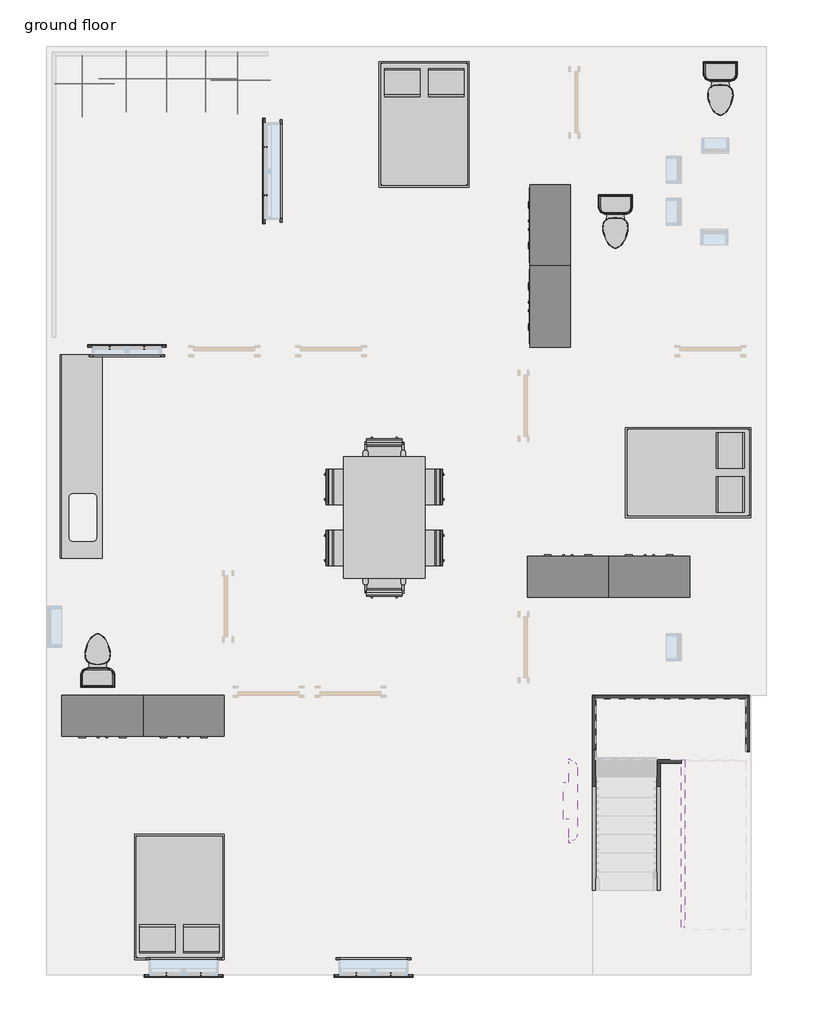
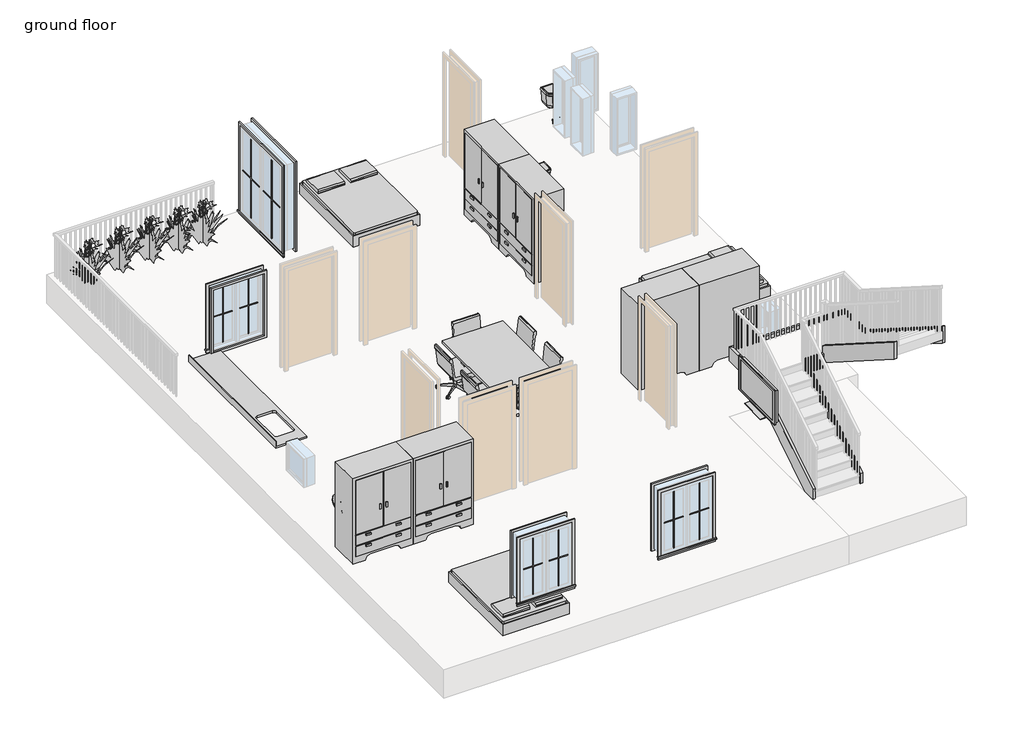
# One storey, part 3 of 3: 18 furniture elements, 16 proxies, 8 members, 5 geographic elements, 3 flow terminals.
"""IFC4 building model written with IfcOpenShell, lengths in millimetres."""

from ifc_helpers import new_model, si_unit, frame, origin, place, context, project, spatial, polyline, outline, extrude, faceted_brep, transform, mapped, element, save
from components import muntin_pattern_2x2_muntin_pattern_2x2_bff912c5, muntin_pattern_2x2_muntin_pattern_2x2_c2194282, muntin_pattern_2x2_muntin_pattern_2x2_88bf7f41, muntin_pattern_2x2_muntin_pattern_2x2_3dfd0a47, trim_window_exterior_flat_with_sill_e04b3088, trim_window_exterior_flat_with_sill_4930676f, trim_window_interior_flat_picture_frame_2a7685fe, trim_window_interior_flat_picture_frame_dd064338, toilet_domestic_3d_toilet_domestic_3d_ba6479b0, toilet_domestic_3d_toilet_domestic_3d_30431060, toilet_domestic_3d_toilet_domestic_3d_9ecb9d01, toilet_domestic_3d_toilet_domestic_3d_e67c3c64, furniture_b58f7881, chair_task_chair_task_b7f3823b, chair_task_arms_chair_task_arms_fa5a08ef, furniture_771c7099, furniture_0b81fedb, furniture_0bcc43ae, furniture_82e269c4, rpc_plant_tropical_55f6ff97

model = new_model("IFC4")

# Units and contexts
model_context = context("Model", 3, world=origin())
ifc_project = project(units=[si_unit("LENGTHUNIT", "METRE", prefix="MILLI")], contexts=[model_context])

# Site, building, storey
site = spatial("IfcSite", under=ifc_project)
building = spatial("IfcBuilding", under=site)
storey = spatial("IfcBuildingStorey", under=building, Name="ground floor", Elevation=609.6)

# Proxies
placement = place(None, origin())
muntin_pattern_2x2_muntin_pattern_2x2_shape = muntin_pattern_2x2_muntin_pattern_2x2_bff912c5(model_context)
element("IfcBuildingElementProxy", 1, Name="Muntin Pattern_2x2 : Muntin Pattern_2x2", ObjectType="Muntin Pattern_2x2 : Muntin Pattern_2x2", at=placement, inside=storey, context=model_context, shape_type="MappedRepresentation", body=[
    mapped(muntin_pattern_2x2_muntin_pattern_2x2_shape, transform((-4824.2248597, 10579.5632925, 1593.85), x_axis=(0.0, 1.0, 0.0), y_axis=(-1.0, 0.0, 0.0), z_axis=(0.0, 0.0, 1.0))),
])
muntin_pattern_2x2_muntin_pattern_2x2_2_shape = muntin_pattern_2x2_muntin_pattern_2x2_c2194282(model_context)
element("IfcBuildingElementProxy", 2, Name="Muntin Pattern_2x2 : Muntin Pattern_2x2", ObjectType="Muntin Pattern_2x2 : Muntin Pattern_2x2", at=placement, inside=storey, context=model_context, shape_type="MappedRepresentation", body=[
    mapped(muntin_pattern_2x2_muntin_pattern_2x2_2_shape, transform((-4824.2248597, 11300.2882925, 1593.85), x_axis=(0.0, -1.0, 0.0), y_axis=(1.0, 0.0, 0.0), z_axis=(0.0, 0.0, 1.0))),
])
muntin_pattern_2x2_muntin_pattern_2x2_3_shape = muntin_pattern_2x2_muntin_pattern_2x2_88bf7f41(model_context)
element("IfcBuildingElementProxy", 3, Name="Muntin Pattern_2x2 : Muntin Pattern_2x2", ObjectType="Muntin Pattern_2x2 : Muntin Pattern_2x2", at=placement, inside=storey, context=model_context, shape_type="MappedRepresentation", body=[
    mapped(muntin_pattern_2x2_muntin_pattern_2x2_3_shape, transform((-7162.6123597, 8288.8007925, 1593.85), x_axis=(1.0, 0.0, 0.0), y_axis=(0.0, 1.0, 0.0), z_axis=(0.0, 0.0, 1.0))),
])
element("IfcBuildingElementProxy", 4, Name="Muntin Pattern_2x2 : Muntin Pattern_2x2", ObjectType="Muntin Pattern_2x2 : Muntin Pattern_2x2", at=placement, inside=storey, context=model_context, shape_type="MappedRepresentation", body=[
    mapped(muntin_pattern_2x2_muntin_pattern_2x2_3_shape, transform((-5794.1873597, -1102.8492075, 1593.85), x_axis=(-1.0, 0.0, 0.0), y_axis=(0.0, -1.0, 0.0), z_axis=(0.0, 0.0, 1.0))),
])
element("IfcBuildingElementProxy", 5, Name="Muntin Pattern_2x2 : Muntin Pattern_2x2", ObjectType="Muntin Pattern_2x2 : Muntin Pattern_2x2", at=placement, inside=storey, context=model_context, shape_type="MappedRepresentation", body=[
    mapped(muntin_pattern_2x2_muntin_pattern_2x2_3_shape, transform((-2946.0873597, -1102.8492075, 1593.85), x_axis=(-1.0, 0.0, 0.0), y_axis=(0.0, -1.0, 0.0), z_axis=(0.0, 0.0, 1.0))),
])
muntin_pattern_2x2_muntin_pattern_2x2_4_shape = muntin_pattern_2x2_muntin_pattern_2x2_3dfd0a47(model_context)
element("IfcBuildingElementProxy", 6, Name="Muntin Pattern_2x2 : Muntin Pattern_2x2", ObjectType="Muntin Pattern_2x2 : Muntin Pattern_2x2", at=placement, inside=storey, context=model_context, shape_type="MappedRepresentation", body=[
    mapped(muntin_pattern_2x2_muntin_pattern_2x2_4_shape, transform((-6645.0873597, 8288.8007925, 1593.85), x_axis=(-1.0, 0.0, 0.0), y_axis=(0.0, -1.0, 0.0), z_axis=(0.0, 0.0, 1.0))),
])
element("IfcBuildingElementProxy", 7, Name="Muntin Pattern_2x2 : Muntin Pattern_2x2", ObjectType="Muntin Pattern_2x2 : Muntin Pattern_2x2", at=placement, inside=storey, context=model_context, shape_type="MappedRepresentation", body=[
    mapped(muntin_pattern_2x2_muntin_pattern_2x2_4_shape, transform((-6311.7123597, -1102.8492075, 1593.85), x_axis=(1.0, 0.0, 0.0), y_axis=(0.0, 1.0, 0.0), z_axis=(0.0, 0.0, 1.0))),
])
element("IfcBuildingElementProxy", 8, Name="Muntin Pattern_2x2 : Muntin Pattern_2x2", ObjectType="Muntin Pattern_2x2 : Muntin Pattern_2x2", at=placement, inside=storey, context=model_context, shape_type="MappedRepresentation", body=[
    mapped(muntin_pattern_2x2_muntin_pattern_2x2_4_shape, transform((-3463.6123597, -1102.8492075, 1593.85), x_axis=(1.0, 0.0, 0.0), y_axis=(0.0, 1.0, 0.0), z_axis=(0.0, 0.0, 1.0))),
])
trim_window_exterior_flat_with_sill_shape = trim_window_exterior_flat_with_sill_e04b3088(model_context)
element("IfcBuildingElementProxy", 9, Name="Trim-Window-Exterior-Flat : with Sill", ObjectType="Trim-Window-Exterior-Flat : with Sill", at=placement, inside=storey, context=model_context, shape_type="MappedRepresentation", body=[
    mapped(trim_window_exterior_flat_with_sill_shape, transform((-4833.7498597, 10939.9257925, 3352.8), x_axis=(0.0, -1.0, 0.0), y_axis=(0.0, 0.0, 1.0), z_axis=(-1.0, 0.0, 0.0))),
])
trim_window_exterior_flat_with_sill_2_shape = trim_window_exterior_flat_with_sill_4930676f(model_context)
element("IfcBuildingElementProxy", 10, Name="Trim-Window-Exterior-Flat : with Sill", ObjectType="Trim-Window-Exterior-Flat : with Sill", at=placement, inside=storey, context=model_context, shape_type="MappedRepresentation", body=[
    mapped(trim_window_exterior_flat_with_sill_2_shape, transform((-6903.8498597, 8298.3257925, 2870.2), x_axis=(-1.0, 0.0, 0.0), y_axis=(0.0, 0.0, 1.0), z_axis=(0.0, 1.0, 0.0))),
])
element("IfcBuildingElementProxy", 11, Name="Trim-Window-Exterior-Flat : with Sill", ObjectType="Trim-Window-Exterior-Flat : with Sill", at=placement, inside=storey, context=model_context, shape_type="MappedRepresentation", body=[
    mapped(trim_window_exterior_flat_with_sill_2_shape, transform((-6052.9498597, -1112.3742075, 2870.2), x_axis=(1.0, 0.0, 0.0), y_axis=(0.0, 0.0, 1.0), z_axis=(0.0, -1.0, 0.0))),
])
element("IfcBuildingElementProxy", 12, Name="Trim-Window-Exterior-Flat : with Sill", ObjectType="Trim-Window-Exterior-Flat : with Sill", at=placement, inside=storey, context=model_context, shape_type="MappedRepresentation", body=[
    mapped(trim_window_exterior_flat_with_sill_2_shape, transform((-3204.8498597, -1112.3742075, 2870.2), x_axis=(1.0, 0.0, 0.0), y_axis=(0.0, 0.0, 1.0), z_axis=(0.0, -1.0, 0.0))),
])
trim_window_interior_flat_picture_frame_shape = trim_window_interior_flat_picture_frame_2a7685fe(model_context)
element("IfcBuildingElementProxy", 13, Name="Trim-Window-Interior-Flat : Picture Frame", ObjectType="Trim-Window-Interior-Flat : Picture Frame", at=placement, inside=storey, context=model_context, shape_type="MappedRepresentation", body=[
    mapped(trim_window_interior_flat_picture_frame_shape, transform((-4605.1498597, 10939.9257925, 3352.8), x_axis=(0.0, 1.0, 0.0), y_axis=(0.0, 0.0, 1.0), z_axis=(1.0, 0.0, 0.0))),
])
trim_window_interior_flat_picture_frame_2_shape = trim_window_interior_flat_picture_frame_dd064338(model_context)
element("IfcBuildingElementProxy", 14, Name="Trim-Window-Interior-Flat : Picture Frame", ObjectType="Trim-Window-Interior-Flat : Picture Frame", at=placement, inside=storey, context=model_context, shape_type="MappedRepresentation", body=[
    mapped(trim_window_interior_flat_picture_frame_2_shape, transform((-6903.8498597, 8184.0257925, 2870.2), x_axis=(1.0, 0.0, 0.0), y_axis=(0.0, 0.0, 1.0), z_axis=(0.0, -1.0, 0.0))),
])
element("IfcBuildingElementProxy", 15, Name="Trim-Window-Interior-Flat : Picture Frame", ObjectType="Trim-Window-Interior-Flat : Picture Frame", at=placement, inside=storey, context=model_context, shape_type="MappedRepresentation", body=[
    mapped(trim_window_interior_flat_picture_frame_2_shape, transform((-6052.9498597, -883.7742075, 2870.2), x_axis=(-1.0, 0.0, 0.0), y_axis=(0.0, 0.0, 1.0), z_axis=(0.0, 1.0, 0.0))),
])
element("IfcBuildingElementProxy", 16, Name="Trim-Window-Interior-Flat : Picture Frame", ObjectType="Trim-Window-Interior-Flat : Picture Frame", at=placement, inside=storey, context=model_context, shape_type="MappedRepresentation", body=[
    mapped(trim_window_interior_flat_picture_frame_2_shape, transform((-3204.8498597, -883.7742075, 2870.2), x_axis=(-1.0, 0.0, 0.0), y_axis=(0.0, 0.0, 1.0), z_axis=(0.0, 1.0, 0.0))),
])

# Flow terminals
toilet_domestic_3d_toilet_domestic_3d_shape = toilet_domestic_3d_toilet_domestic_3d_ba6479b0(model_context)
toilet_domestic_3d_toilet_domestic_3d_2_shape = toilet_domestic_3d_toilet_domestic_3d_30431060(model_context)
element("IfcFlowTerminal", 17, ObjectType="Toilet-Domestic-3D : Toilet-Domestic-3D", at=placement, inside=storey, context=model_context, shape_type="MappedRepresentation", body=[
    mapped(toilet_domestic_3d_toilet_domestic_3d_shape, transform((424.0501403, 10089.0257925, 609.6), x_axis=(1.0, 0.0, 0.0), y_axis=(0.0, 1.0, 0.0), z_axis=(0.0, 0.0, 1.0))),
    mapped(toilet_domestic_3d_toilet_domestic_3d_2_shape, transform((424.0501403, 10089.0257925, 609.6), x_axis=(1.0, 0.0, 0.0), y_axis=(0.0, 1.0, 0.0), z_axis=(0.0, 0.0, 1.0))),
])
element("IfcFlowTerminal", 18, ObjectType="Toilet-Domestic-3D : Toilet-Domestic-3D", at=placement, inside=storey, context=model_context, shape_type="MappedRepresentation", body=[
    mapped(toilet_domestic_3d_toilet_domestic_3d_shape, transform((1998.8501403, 12083.5297652, 609.6), x_axis=(1.0, 0.0, 0.0), y_axis=(0.0, 1.0, 0.0), z_axis=(0.0, 0.0, 1.0))),
    mapped(toilet_domestic_3d_toilet_domestic_3d_2_shape, transform((1998.8501403, 12083.5297652, 609.6), x_axis=(1.0, 0.0, 0.0), y_axis=(0.0, 1.0, 0.0), z_axis=(0.0, 0.0, 1.0))),
])
toilet_domestic_3d_toilet_domestic_3d_3_shape = toilet_domestic_3d_toilet_domestic_3d_9ecb9d01(model_context)
toilet_domestic_3d_toilet_domestic_3d_4_shape = toilet_domestic_3d_toilet_domestic_3d_e67c3c64(model_context)
element("IfcFlowTerminal", 19, ObjectType="Toilet-Domestic-3D : Toilet-Domestic-3D", at=placement, inside=storey, context=model_context, shape_type="MappedRepresentation", body=[
    mapped(toilet_domestic_3d_toilet_domestic_3d_3_shape, transform((-7342.9058187, 3694.2738062, 609.6), x_axis=(1.0, 0.0, 0.0), y_axis=(0.0, 1.0, 0.0), z_axis=(0.0, 0.0, 1.0))),
    mapped(toilet_domestic_3d_toilet_domestic_3d_4_shape, transform((-7342.9058187, 3694.2738062, 609.6), x_axis=(1.0, 0.0, 0.0), y_axis=(0.0, 1.0, 0.0), z_axis=(0.0, 0.0, 1.0))),
])

# Furniture
furniture_shape = furniture_b58f7881(model_context)
element("IfcFurniture", 20, ObjectType="Bed-Box : Double 53\" x 74\"", at=placement, inside=storey, context=model_context, shape_type="MappedRepresentation", body=[
    mapped(furniture_shape, transform((-2785.3023187, 11872.8553007, 609.6), x_axis=(1.0, 0.0, 0.0), y_axis=(0.0, 1.0, 0.0), z_axis=(0.0, 0.0, 1.0))),
])
element("IfcFurniture", 21, ObjectType="Bed-Box : Double 53\" x 74\"", at=placement, inside=storey, context=model_context, shape_type="MappedRepresentation", body=[
    mapped(furniture_shape, transform((1750.6796485, 6757.8782516, 609.6), x_axis=(0.0, -1.0, 0.0), y_axis=(1.0, 0.0, 0.0), z_axis=(0.0, 0.0, 1.0))),
])
element("IfcFurniture", 22, ObjectType="Bed-Box : Double 53\" x 74\"", at=placement, inside=storey, context=model_context, shape_type="MappedRepresentation", body=[
    mapped(furniture_shape, transform((-5777.2974007, -178.4037157, 609.6), x_axis=(-1.0, 0.0, 0.0), y_axis=(0.0, -1.0, 0.0), z_axis=(0.0, 0.0, 1.0))),
])
chair_task_chair_task_shape = chair_task_chair_task_b7f3823b(model_context)
element("IfcFurniture", 23, ObjectType="Chair-Task : Chair-Task", at=placement, inside=storey, context=model_context, shape_type="MappedRepresentation", body=[
    mapped(chair_task_chair_task_shape, transform((-3671.5957614, 6343.8166122, 609.6), x_axis=(0.0, -1.0, 0.0), y_axis=(1.0, 0.0, 0.0), z_axis=(0.0, 0.0, 1.0))),
])
element("IfcFurniture", 24, ObjectType="Chair-Task : Chair-Task", at=placement, inside=storey, context=model_context, shape_type="MappedRepresentation", body=[
    mapped(chair_task_chair_task_shape, transform((-2414.5039581, 6061.8349729, 609.6), x_axis=(0.0, 1.0, 0.0), y_axis=(-1.0, 0.0, 0.0), z_axis=(0.0, 0.0, 1.0))),
])
element("IfcFurniture", 25, ObjectType="Chair-Task : Chair-Task", at=placement, inside=storey, context=model_context, shape_type="MappedRepresentation", body=[
    mapped(chair_task_chair_task_shape, transform((-3671.5957614, 5429.4166122, 609.6), x_axis=(0.0, -1.0, 0.0), y_axis=(1.0, 0.0, 0.0), z_axis=(0.0, 0.0, 1.0))),
])
element("IfcFurniture", 26, ObjectType="Chair-Task : Chair-Task", at=placement, inside=storey, context=model_context, shape_type="MappedRepresentation", body=[
    mapped(chair_task_chair_task_shape, transform((-2414.5039581, 5147.4349729, 609.6), x_axis=(0.0, 1.0, 0.0), y_axis=(-1.0, 0.0, 0.0), z_axis=(0.0, 0.0, 1.0))),
])
chair_task_arms_chair_task_arms_shape = chair_task_arms_chair_task_arms_fa5a08ef(model_context)
element("IfcFurniture", 27, ObjectType="Chair-Task Arms : Chair-Task Arms", at=placement, inside=storey, context=model_context, shape_type="MappedRepresentation", body=[
    mapped(chair_task_arms_chair_task_arms_shape, transform((-3184.0406794, 4812.2798909, 609.6), x_axis=(1.0, 0.0, 0.0), y_axis=(0.0, 1.0, 0.0), z_axis=(0.0, 0.0, 1.0))),
])
element("IfcFurniture", 28, ObjectType="Chair-Task Arms : Chair-Task Arms", at=placement, inside=storey, context=model_context, shape_type="MappedRepresentation", body=[
    mapped(chair_task_arms_chair_task_arms_shape, transform((-2902.05904, 6678.9716942, 609.6), x_axis=(-1.0, 0.0, 0.0), y_axis=(0.0, -1.0, 0.0), z_axis=(0.0, 0.0, 1.0))),
])
furniture_2_shape = furniture_771c7099(model_context)
element("IfcFurniture", 29, ObjectType="Counter Top w Sink Hole : 24\" Depth", at=placement, inside=storey, context=model_context, shape_type="MappedRepresentation", body=[
    mapped(furniture_2_shape, transform((-7907.1498597, 6336.4880876, 609.6), x_axis=(0.0, 1.0, 0.0), y_axis=(-1.0, 0.0, 0.0), z_axis=(0.0, 0.0, 1.0))),
])
furniture_3_shape = furniture_0b81fedb(model_context)
element("IfcFurniture", 30, ObjectType="TV - Flat Screen : 50\"", at=placement, inside=storey, context=model_context, shape_type="MappedRepresentation", body=[
    mapped(furniture_3_shape, transform((-205.9884834, 1493.5704198, 1828.8), x_axis=(0.0, -1.0, 0.0), y_axis=(1.0, 0.0, 0.0), z_axis=(0.0, 0.0, 1.0))),
])
furniture_4_shape = furniture_0bcc43ae(model_context)
element("IfcFurniture", 31, ObjectType="Table-Conference2 w Chairs : 48\" x 144\"", at=placement, inside=storey, context=model_context, shape_type="MappedRepresentation", body=[
    mapped(furniture_4_shape, transform((-3043.0498597, 5745.6257925, 609.6), x_axis=(0.0, 1.0, 0.0), y_axis=(-1.0, 0.0, 0.0), z_axis=(0.0, 0.0, 1.0))),
])
furniture_5_shape = furniture_82e269c4(model_context)
element("IfcFurniture", 32, ObjectType="Wardrobe : 48\" x 72\" x 24\"", at=placement, inside=storey, context=model_context, shape_type="MappedRepresentation", body=[
    mapped(furniture_5_shape, transform((29.8889499, 8638.7325327, 609.6), x_axis=(0.0, -1.0, 0.0), y_axis=(1.0, 0.0, 0.0), z_axis=(0.0, 0.0, 1.0))),
])
element("IfcFurniture", 33, ObjectType="Wardrobe : 48\" x 72\" x 24\"", at=placement, inside=storey, context=model_context, shape_type="MappedRepresentation", body=[
    mapped(furniture_5_shape, transform((29.8889499, 9857.9325327, 609.6), x_axis=(0.0, -1.0, 0.0), y_axis=(1.0, 0.0, 0.0), z_axis=(0.0, 0.0, 1.0))),
])
element("IfcFurniture", 34, ObjectType="Wardrobe : 48\" x 72\" x 24\"", at=placement, inside=storey, context=model_context, shape_type="MappedRepresentation", body=[
    mapped(furniture_5_shape, transform((-556.3431196, 4272.886983, 609.6), x_axis=(-1.0, 0.0, 0.0), y_axis=(0.0, -1.0, 0.0), z_axis=(0.0, 0.0, 1.0))),
])
element("IfcFurniture", 35, ObjectType="Wardrobe : 48\" x 72\" x 24\"", at=placement, inside=storey, context=model_context, shape_type="MappedRepresentation", body=[
    mapped(furniture_5_shape, transform((662.8568804, 4272.886983, 609.6), x_axis=(-1.0, 0.0, 0.0), y_axis=(0.0, -1.0, 0.0), z_axis=(0.0, 0.0, 1.0))),
])
element("IfcFurniture", 36, ObjectType="Wardrobe : 48\" x 72\" x 24\"", at=placement, inside=storey, context=model_context, shape_type="MappedRepresentation", body=[
    mapped(furniture_5_shape, transform((-7002.9565999, 3357.5646021, 609.6), x_axis=(1.0, 0.0, 0.0), y_axis=(0.0, 1.0, 0.0), z_axis=(0.0, 0.0, 1.0))),
])
element("IfcFurniture", 37, ObjectType="Wardrobe : 48\" x 72\" x 24\"", at=placement, inside=storey, context=model_context, shape_type="MappedRepresentation", body=[
    mapped(furniture_5_shape, transform((-5783.7565999, 3357.5646021, 609.6), x_axis=(1.0, 0.0, 0.0), y_axis=(0.0, 1.0, 0.0), z_axis=(0.0, 0.0, 1.0))),
])

# Geographic elements
rpc_plant_tropical_shape = rpc_plant_tropical_55f6ff97(model_context)
element("IfcGeographicElement", 38, ObjectType="RPC Plant - Tropical", at=placement, inside=storey, context=model_context, shape_type="MappedRepresentation", body=[
    mapped(rpc_plant_tropical_shape, transform((-7576.9498597, 12248.0257925, 609.6), x_axis=(1.0, 0.0, 0.0), y_axis=(0.0, 1.0, 0.0), z_axis=(0.0, 0.0, 1.0))),
])
element("IfcGeographicElement", 39, ObjectType="RPC Plant - Tropical", at=placement, inside=storey, context=model_context, shape_type="MappedRepresentation", body=[
    mapped(rpc_plant_tropical_shape, transform((-5240.1498597, 12298.8257925, 609.6), x_axis=(1.0, 0.0, 0.0), y_axis=(0.0, 1.0, 0.0), z_axis=(0.0, 0.0, 1.0))),
])
element("IfcGeographicElement", 40, ObjectType="RPC Plant - Tropical", at=placement, inside=storey, context=model_context, shape_type="MappedRepresentation", body=[
    mapped(rpc_plant_tropical_shape, transform((-6916.5498597, 12324.2257925, 609.6), x_axis=(1.0, 0.0, 0.0), y_axis=(0.0, 1.0, 0.0), z_axis=(0.0, 0.0, 1.0))),
])
element("IfcGeographicElement", 41, ObjectType="RPC Plant - Tropical", at=placement, inside=storey, context=model_context, shape_type="MappedRepresentation", body=[
    mapped(rpc_plant_tropical_shape, transform((-6306.9498597, 12324.2257925, 609.6), x_axis=(1.0, 0.0, 0.0), y_axis=(0.0, 1.0, 0.0), z_axis=(0.0, 0.0, 1.0))),
])
element("IfcGeographicElement", 42, ObjectType="RPC Plant - Tropical", at=placement, inside=storey, context=model_context, shape_type="MappedRepresentation", body=[
    mapped(rpc_plant_tropical_shape, transform((-5722.7498597, 12324.2257925, 609.6), x_axis=(1.0, 0.0, 0.0), y_axis=(0.0, 1.0, 0.0), z_axis=(0.0, 0.0, 1.0))),
])

# Members
element("IfcMember", 43, ObjectType="Stringer - 2\" Width", at=placement, inside=storey, context=model_context, shape_type="SweptSolid", body=[
    extrude(outline(polyline([(157.6257925, 609.6), (157.6257925, 824.6106437), (2174.694781, 2108.2), (2263.4527505, 1803.4), (387.4813219, 609.6), (157.6257925, 609.6)])), frame((81.1501403, 0.0, 0.0), z_axis=(1.0, 0.0, 0.0), x_axis=(0.0, 1.0, 0.0)), (0.0, 0.0, 1.0), 50.8),
])
element("IfcMember", 44, ObjectType="Stringer - 2\" Width", at=placement, inside=storey, context=model_context, shape_type="SweptSolid", body=[
    extrude(outline(polyline([(157.6257925, 609.6), (157.6257925, 824.6106437), (2062.6257925, 2036.883371), (2062.6257925, 1675.6010268), (387.4813219, 609.6), (157.6257925, 609.6)])), frame((1046.3501403, 0.0, 0.0), z_axis=(1.0, 0.0, 0.0), x_axis=(0.0, 1.0, 0.0)), (0.0, 0.0, 1.0), 50.8),
])
element("IfcMember", 45, ObjectType="Stringer - 2\" Width", at=placement, inside=storey, context=model_context, shape_type="SweptSolid", body=[
    extrude(outline(polyline([(2331.5568041, 2108.2), (2242.7988346, 1803.4), (-401.1742075, 3485.9282995), (-401.1742075, 3847.2106437), (2331.5568041, 2108.2)])), frame((2379.8501403, 0.0, 0.0), z_axis=(1.0, 0.0, 0.0), x_axis=(0.0, 1.0, 0.0)), (0.0, 0.0, 1.0), 50.8),
])
element("IfcMember", 46, ObjectType="Stringer - 2\" Width", at=placement, inside=storey, context=model_context, shape_type="SweptSolid", body=[
    extrude(outline(polyline([(2113.4257925, 2247.0106437), (2113.4257925, 1885.7282995), (-401.1742075, 3485.9282995), (-401.1742075, 3847.2106437), (2113.4257925, 2247.0106437)])), frame((1414.6501403, 0.0, 0.0), z_axis=(1.0, 0.0, 0.0), x_axis=(0.0, 1.0, 0.0)), (0.0, 0.0, 1.0), 50.8),
])
element("IfcMember", 47, ObjectType="Stringer - 2\" Width", at=placement, inside=storey, context=model_context, shape_type="Brep", body=[
    faceted_brep([(2379.8501403, 2331.5568041, 2108.2), (2430.6501403, 2331.5568041, 2108.2), (2430.6501403, 3078.6257925, 2108.2), (2379.8501403, 3027.8257925, 2108.2), (2379.8501403, 2242.7988346, 1803.4), (2379.8501403, 3027.8257925, 1803.4), (2430.6501403, 2242.7988346, 1803.4), (2430.6501403, 3078.6257925, 1803.4)], [[[0, 1, 2, 3]], [[4, 0, 3, 5]], [[6, 4, 5, 7]], [[1, 6, 7, 2]], [[1, 0, 4, 6]], [[2, 7, 5, 3]]]),
])
element("IfcMember", 48, ObjectType="Stringer - 2\" Width", at=placement, inside=storey, context=model_context, shape_type="SweptSolid", body=[
    extrude(outline(polyline([(2430.6501403, 3078.6257925), (2379.8501403, 3027.8257925), (131.9501403, 3027.8257925), (81.1501403, 3078.6257925), (2430.6501403, 3078.6257925)])), frame((0.0, 0.0, 1803.4), z_axis=(0.0, 0.0, 1.0), x_axis=(1.0, 0.0, 0.0)), (0.0, 0.0, 1.0), 304.8),
])
element("IfcMember", 49, ObjectType="Stringer - 2\" Width", at=placement, inside=storey, context=model_context, shape_type="Brep", body=[
    faceted_brep([(131.9501403, 3027.8257925, 2108.2), (81.1501403, 3078.6257925, 2108.2), (81.1501403, 2174.694781, 2108.2), (131.9501403, 2174.694781, 2108.2), (131.9501403, 3027.8257925, 1803.4), (131.9501403, 2263.4527505, 1803.4), (81.1501403, 3078.6257925, 1803.4), (81.1501403, 2263.4527505, 1803.4)], [[[0, 1, 2, 3]], [[4, 0, 3, 5]], [[6, 4, 5, 7]], [[1, 6, 7, 2]], [[1, 0, 4, 6]], [[2, 7, 5, 3]]]),
])
element("IfcMember", 50, ObjectType="Stringer - 2\" Width", at=placement, inside=storey, context=model_context, shape_type="SweptSolid", body=[
    extrude(outline(polyline([(1046.3501403, 2062.6257925), (1046.3501403, 2113.4257925), (1414.6501403, 2113.4257925), (1414.6501403, 2062.6257925), (1046.3501403, 2062.6257925)])), frame((0.0, 0.0, 1803.4), z_axis=(0.0, 0.0, 1.0), x_axis=(1.0, 0.0, 0.0)), (0.0, 0.0, 1.0), 304.8),
])

save(model, "model.ifc")

# Revit data of these elements
# Type "Muntin Pattern_2x2 : Muntin Pattern_2x2"
#   Width [instance default] = 4' - 0"
#   Thickness = 0' - 0 1/2"
#   Height [instance default] = 4' - 0"
#   Distance = 0' - 0 3/4"
#   Interior Material [instance default] = none
#   Exterior Material [instance default] = none
#   Default Elevation = 0
# Type "Trim-Window-Exterior-Flat : with Sill"
#   Trim Width = 0' - 2 1/4"
#   Trim Thickness_Picture Frame = 0' - 1 1/4"
#   Trim Thickness_with Sill = 0' - 0 3/4"
#   Sill Thickness = 0' - 1 1/4"
#   Opening Width [instance default] = 2' - 0"
#   Opening Height [instance default] = 3' - 0"
#   Default Elevation = 4' - 0"
#   Sill = yes
#   Picture Frame = no
#   Trim Material [instance default] = none
# Type "Trim-Window-Interior-Flat : Picture Frame"
#   Trim Thickness_Picture Frame = 0' - 1 1/4"
#   Trim Width = 0' - 2 1/4"
#   Trim Thickness_with Sill = 0' - 0 3/4"
#   Sill Thickness = 0' - 1 1/4"
#   Opening Width [instance default] = 2' - 0"
#   Opening Height [instance default] = 3' - 0"
#   Default Elevation = 4' - 0"
#   Sill = no
#   Picture Frame = yes
#   Trim Material [instance default] = none
# Type "Toilet-Domestic-3D : Toilet-Domestic-3D"
#   Assembly Code = "D2010110"
#   Toilet - Bowl/Basin Material = Porcelain, Linen
#   Toilet - Seat Material = Laminate, Linen, Matte
#   Default Elevation = 0
# Type "Bed-Box : Double 53\" x 74\""
#   Assembly Code = "E2020200"
#   Length = 6' - 2"
#   Width = 4' - 5"
#   Frame Material = Birch
#   Mattress Material = Linen, White
#   Default Elevation = 0
# Type "Chair-Task : Chair-Task"
#   Assembly Code = "E2020200"
#   Base Material = Plastic - Black
#   Caster Material = Plastic - Black
#   Seat/Back Material = Textile - Slate Blue
#   Default Elevation = 0
# Type "Chair-Task Arms : Chair-Task Arms"
#   Assembly Code = "E2020200"
#   Base Material = Plastic - Black
#   Caster Material = Plastic - Black
#   Seat/Back Material = Textile - Slate Blue
#   Default Elevation = 0
# Type "Counter Top w Sink Hole : 24\" Depth"
#   Assembly Code = "C1030400"
#   Counter Thickness = 0' - 1 1/2"
#   Depth = 2' - 1"
#   Height = 3' - 0"
#   Length [instance default] = 8' - 0"
#   Sink Location [instance default] = 2' - 0"
#   Sink Location To Wall [instance default] = 0' - 6"
#   Sink Opening Depth [instance default] = 1' - 3"
#   Sink Opening Width [instance default] = 2' - 3"
#   Counter Top Material = none
#   Default Elevation = 0
# Type "TV - Flat Screen : 50\""
#   SinAng = 0' - 0.0193"
#   L = 3' - 7.57782"
#   H = 2' - 0.51477"
#   Thickness = 0' - 4.33071"
#   Diagonal = 4' - 2"
#   CosAng = 0' - 0.03431"
#   Stand [instance default] = yes
#   Default Elevation = 0
# Type "Table-Conference2 w Chairs : 48\" x 144\""
#   Assembly Code = "E2020200"
#   Description = "Seating 12-14"
#   Height = 2' - 6"
#   Length = 6' - 0"
#   Width = 4' - 0"
#   Number Of Chairs One Side = 2
#   Number Of Chairs = 6
#   Material = Wood - Cherry
#   Default Elevation = 0
# Type "Wardrobe : 48\" x 72\" x 24\""
#   Assembly Code = "E2020200"
#   Depth = 2' - 0"
#   Height = 6' - 0"
#   Width = 4' - 0"
#   Material = Wood - Mahogany
#   Default Elevation = 0
# Type "RPC Plant - Tropical"
#   built-in parameter 1005198 = "{2, 15},{39, RPC-16-FWM5-GM7X-C67P-4000-ST1L-LVER-AU},{1, 0},{1, 0},{2, 35},{1, 8},{5, Color},{1, 0},{1, 0},{3, 0.8},{3, 0.8},{3, 0.8},{1, 8},{7, BBoxMin},{1, 0},{1, 0},{1, 0},{1, 0},{1, 0},{1, 8},{7, BBoxMax},{1, 0},{1, 0},{1, 0},{1, 0},{1, 0},{2, 11},{9, RPCTypeId},{1, 0},{1, 0},{39, RPC-16-FWM5-GM7X-C67P-4000-ST1L-LVER-AU},{1, 6},{14, RPCPlantHeight},{1, 0},{1, 0},{1, 3},{2, 11},{7, keyword},{1, 0},{1, 0},{99, :Geometry:RPC:Crane Lily:strelitzia:reinae:crane lily:plants:shrub:flower:tropical:bird-of-paradise},{2, 11},{8, category},{1, 0},{1, 0},{17, :Shrubs [General]},{2, 11},{12, LocalizedUID},{1, 0},{1, 0},{10, Crane Lily},{2, 14},{6, Height},{1, 0},{1, 0},{1, 3},{1, 2},{16, Cast Reflections},{1, 0},{1, 0},{1, 0},{1, 2},{12, Cast Shadows},{1, 0},{1, 0},{1, 1},{1, 2},{9, Lock View},{1, 0},{1, 0},{1, 0},{1, 4},{5, ViewC},{1, 0},{1, 0},{1, 0},{2, 11},{20, AdvancedUIDefinition},{1, 0},{1, 0},{0, },{2, 11},{10, AssetLibID},{1, 0},{1, 0},{36, 4D3F6E72-3F99-4203-98E9-AF80B3C7A7A4},{2, 11},{10, BaseSchema},{1, 0},{1, 0},{9, RPCSchema},{2, 11},{12, ExchangeGUID},{1, 0},{1, 0},{0, },{1, 2},{6, Hidden},{1, 0},{1, 0},{1, 0},{1, 4},{11, RPCCategory},{1, 0},{1, 0},{1, 0},{2, 11},{8, RPCImage},{1, 0},{1, 0},{0, },{1, 4},{13, SchemaVersion},{1, 0},{1, 0},{1, 4},{2, 11},{12, UIDefinition},{1, 0},{1, 0},{0, },{2, 11},{6, UIName},{1, 0},{1, 0},{39, RPC-16-FWM5-GM7X-C67P-4000-ST1L-LVER-AU},{2, 11},{11, VersionGUID},{1, 0},{1, 0},{9, RPCSchema},{2, 11},{9, assettype},{1, 0},{1, 0},{11, RPCGeometry},{2, 11},{11, description},{1, 0},{1, 0},{0, },{2, 11},{9, localname},{1, 0},{1, 0},{3, RPC},{2, 11},{9, localtype},{1, 0},{1, 0},{3, RPC},{1, 4},{8, revision},{1, 0},{1, 0},{1, 1},{2, 11},{9, thumbnail},{1, 0},{1, 0},{0, },{1, 4},{7, version},{1, 0},{1, 0},{1, 1},{1, 2},{20, RPC_Cast Reflections},{1, 0},{1, 0},{1, 1},{1, 2},{16, RPC_Cast Shadows},{1, 0},{1, 0},{1, 1},{1, 2},{13, RPC_Lock View},{1, 0},{1, 0},{1, 0},{1, 4},{9, RPC_ViewC},{1, 0},{1, 0},{1, 0},{21, assetlibrary_base.fbx},{1, 5},"
#   built-in parameter 1005195 = "RPC-16-FWM5-GM7X-C67P-4000-ST1L-LVER-AU"
#   Assembly Code = "G2050500"
#   Height = 3' - 0"
#   Default Elevation = 0
# Elements 1, 2 (IfcBuildingElementProxy, "Muntin Pattern_2x2 : Muntin Pattern_2x2")
#   Width = 1' - 11 1/8"
#   Height = 5' - 6 1/2"
#   Interior Material = Wood - Stained
#   Exterior Material = Clad - White
#   Phase Created = New Construction
#   Materials on its faces: "Clad - White", "Wood - Stained"
# Elements 3, 4, 5, 6, 7, 8 (IfcBuildingElementProxy, "Muntin Pattern_2x2 : Muntin Pattern_2x2")
#   Width = 1' - 3 1/8"
#   Height = 3' - 11 1/2"
#   Interior Material = Wood - Stained
#   Exterior Material = Clad - White
#   Phase Created = New Construction
#   Materials on its faces: "Clad - White", "Wood - Stained"
# Element 9 (IfcBuildingElementProxy, "Trim-Window-Exterior-Flat : with Sill")
#   Opening Width = 4' - 9"
#   Opening Height = 6' - 0"
#   Trim Material = Clad - White
#   Phase Created = New Construction
#   Materials on its faces: "Clad - White"
# Elements 10, 11, 12 (IfcBuildingElementProxy, "Trim-Window-Exterior-Flat : with Sill")
#   Opening Width = 3' - 5"
#   Opening Height = 4' - 5"
#   Trim Material = Clad - White
#   Phase Created = New Construction
#   Materials on its faces: "Clad - White"
# Element 13 (IfcBuildingElementProxy, "Trim-Window-Interior-Flat : Picture Frame")
#   Opening Width = 4' - 9"
#   Opening Height = 6' - 0"
#   Trim Material = Wood - Stained
#   Phase Created = New Construction
#   Materials on its faces: "Wood - Stained"
# Elements 14, 15, 16 (IfcBuildingElementProxy, "Trim-Window-Interior-Flat : Picture Frame")
#   Opening Width = 3' - 5"
#   Opening Height = 4' - 5"
#   Trim Material = Wood - Stained
#   Phase Created = New Construction
#   Materials on its faces: "Wood - Stained"
# Element 17 (IfcFlowTerminal, "Toilet-Domestic-3D : Toilet-Domestic-3D")
#   Mark = "4"
#   Phase Created = New Construction
#   Materials on its faces: "Porcelain, Linen", "Laminate, Linen, Matte"
# Element 18 (IfcFlowTerminal, "Toilet-Domestic-3D : Toilet-Domestic-3D")
#   Mark = "5"
#   Phase Created = New Construction
#   Materials on its faces: "Porcelain, Linen", "Laminate, Linen, Matte"
# Element 19 (IfcFlowTerminal, "Toilet-Domestic-3D : Toilet-Domestic-3D")
#   Mark = "3"
#   Phase Created = New Construction
#   Materials on its faces: "Porcelain, Linen", "Laminate, Linen, Matte"
# Elements 20, 21, 22 (IfcFurniture, "Bed-Box : Double 53\" x 74\"")
#   Phase Created = New Construction
#   Materials on its faces: "Birch", "Linen, White"
# Elements 23, 24, 25, 26 (IfcFurniture, "Chair-Task : Chair-Task")
#   Phase Created = New Construction
#   Materials on its faces: "Plastic - Black", "Textile - Slate Blue"
# Elements 27, 28 (IfcFurniture, "Chair-Task Arms : Chair-Task Arms")
#   Phase Created = New Construction
#   Materials on its faces: "Plastic - Black", "Textile - Slate Blue"
# Element 29 (IfcFurniture, "Counter Top w Sink Hole : 24\" Depth")
#   Sink Opening Width = 2' - 3"
#   Sink Opening Depth = 1' - 3"
#   Sink Location To Wall = 0' - 6"
#   Sink Location = 2' - 0"
#   Length = 10' - 0"
#   Phase Created = New Construction
#   Materials on its faces: "Counter Top"
# Element 30 (IfcFurniture, "TV - Flat Screen : 50\"")
#   Stand = yes
#   Phase Created = New Construction
#   Materials on its faces: "TV - Black", "TV - Glass", "TV - Screen"
# Element 31 (IfcFurniture, "Table-Conference2 w Chairs : 48\" x 144\"")
#   Phase Created = New Construction
#   Materials on its faces: "Wood - Cherry"
# Elements 32, 33, 34, 35, 36, 37 (IfcFurniture, "Wardrobe : 48\" x 72\" x 24\"")
#   Phase Created = New Construction
#   Materials on its faces: "Wood - Mahogany"
# Elements 38, 39, 40, 41, 42 (IfcGeographicElement, "RPC Plant - Tropical")
#   Phase Created = New Construction
# Elements 43, 44, 45, 46, 47, 48, 49, 50 (IfcMember, "Stringer - 2\" Width")
#   Phase Created = New Construction
# Materials
#   "Porcelain, Linen": class "Ceramic", colour RGB 249 239 230, transparency 0, Description = "Porcelain, linen", Cost = 0
#   "Laminate, Linen, Matte": class "Plastic", colour RGB 249 239 230, transparency 0, Description = "Plastic Laminate - Linen, Matte", Cost = 0
#   "Birch": class "Wood", colour RGB 224 178 126, transparency 0, Description = "Betula Alleghaniensis", Cost = 0
#   "Linen, White": class "Textile", colour RGB 247 247 239, transparency 0, Description = "Linen, white", Cost = 0
#   "Plastic - Black": colour RGB 0 0 0, transparency 0.7
#   "Textile - Slate Blue": colour RGB 98 102 118, transparency 0
#   "Wood - Cherry": colour RGB 151 75 0, transparency 0
#   "Wood - Mahogany": colour RGB 138 86 45, transparency 0
#   "Clad - White": class "Wood", colour RGB 242 242 238, transparency 0, Cost = 0
#   "Wood - Stained": class "Wood", colour RGB 224 178 126, transparency 0, Cost = 0
#   "Counter Top": class "Wood", colour RGB 226 177 128, transparency 0
#   "TV - Black": colour RGB 49 49 49, transparency 0
#   "TV - Glass": colour RGB 157 157 157, transparency 0.9
#   "TV - Screen": colour RGB 0 0 0, transparency 0
